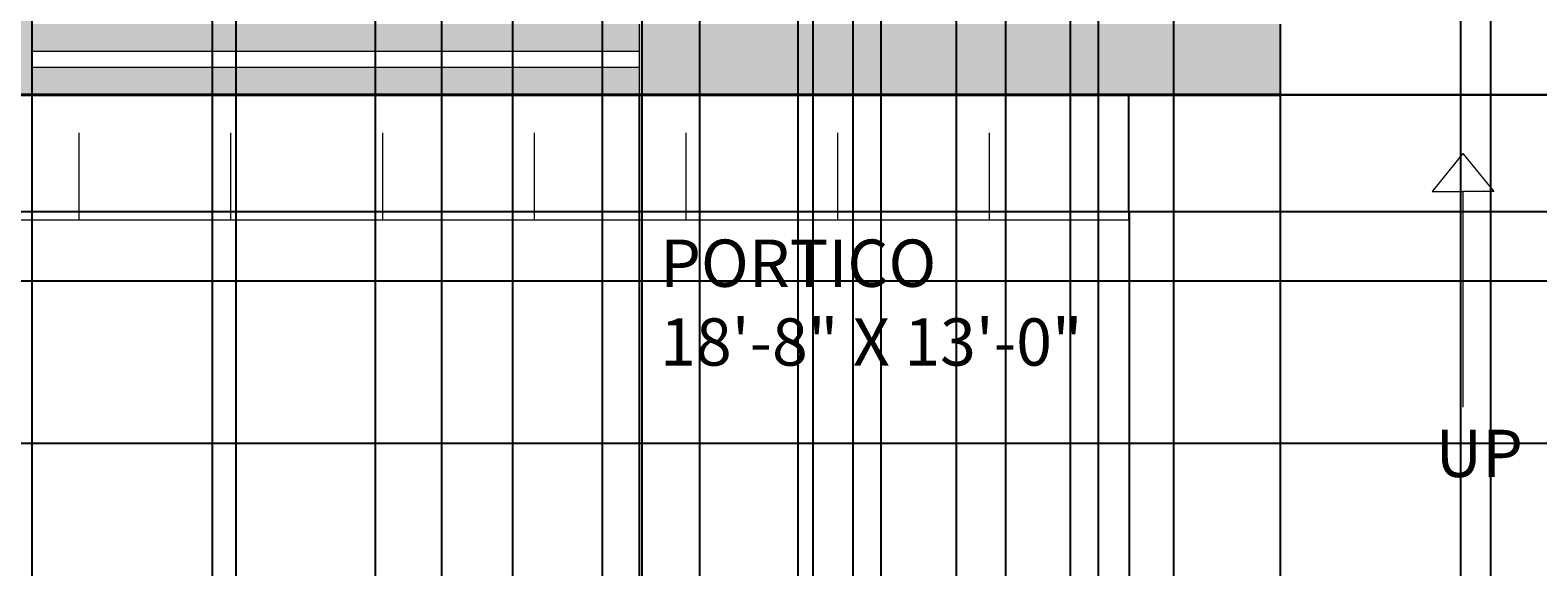
# Model space of a CAD drawing. Units: inches. Extents: x 818 to 1898, y 976 to 2364.
# Tile 22 of 96: x 1207 to 1398, y 1441 to 1509. Entities that reach past the tile are written whole.
import ezdxf

# ---------------------------------------------------------------- set-up
doc = ezdxf.new("R2010")
doc.units = ezdxf.units.IN
doc.header["$LTSCALE"] = 5
doc.header["$MEASUREMENT"] = 0
for name, color, linetype, lineweight in [('A-ANNO-DIMS', 2, 'Continuous', 18), ('A-ANNO-SYMB', 7, 'Continuous', 18), ('A-ANNO-TEXT', 7, 'Continuous', 18), ('A-AREA-IDEN', 7, 'Continuous', 18), ('A-DOOR', 3, 'Continuous', 25), ('A-FLOR-STRS', 7, 'Continuous', 25), ('A-GLAZ', 4, 'Continuous', 18), ('A-WALL', 7, 'Continuous', 40), ('C-PKNG', 8, 'Continuous', 18), ('C-PKNG-PATT', 9, 'Continuous', 9)]:
    doc.layers.add(name, color=color, linetype=linetype, lineweight=lineweight)
doc.layers.add('A-GLAZ-PATT', color=141, linetype='Continuous', lineweight=9, true_color=0xadddf7)
doc.layers.add('A-WALL-PATT', color=251, linetype='Continuous', lineweight=13, true_color=0x636466)
doc.styles.get("Standard").update_dxf_attribs({"font": 'arial.ttf'})
doc.dimstyles.get("Standard").update_dxf_attribs({"dimtxt": 0.18, "dimasz": 0.18, "dimexe": 0.18, "dimexo": 0.0625, "dimgap": 0.09, "dimtad": 0, "dimtih": 1, "dimtoh": 1, "dimdec": 4, "dimzin": 0, "dimdsep": 46, "dimtxsty": 'Standard', "dimcen": 0.09, "dimadec": 0, "dimazin": 0, "dimtfac": 1, "dimtdec": 4, "dimtofl": 0, "dimtmove": 0, "dimatfit": 3, "dimfxl": 1, "dimtolj": 1, "dimtzin": 0, "dimarcsym": 0})
pattern_1 = [(0, (0, 0), (0, 19.25), [14, -5.25]), (90, (0, 0), (-19.25, 1e-15), [14, -5.25])]

# ---------------------------------------------------------------- blocks, each defined once
blk = doc.blocks.new('*D59')
at = {"layer": 'A-ANNO-DIMS', "color": 0, "lineweight": -2, "ltscale": 5, "transparency": 16777216}
for p, q in [((1251.64, 2300.39), (818.03, 2300.39)), ((818.21, 2300.21), (818.21, 1669.95)), ((818.21, 1039.32), (818.21, 1669.59)), ((896.05, 1039.14), (818.03, 1039.14))]:
    blk.add_line(p, q, dxfattribs=at)
at = {"layer": 'A-ANNO-DIMS', "color": 0, "ltscale": 5, "transparency": 16777216}
for points in [[(818.18, 2300.21), (818.24, 2300.21), (818.21, 2300.39)], [(818.18, 1039.32), (818.24, 1039.32), (818.21, 1039.14)]]:
    blk.add_solid(points, dxfattribs=at)
at = {"layer": 'Defpoints', "color": 0, "ltscale": 5, "transparency": 16777216}
for p in [(818.21, 2300.39), (1251.71, 2300.39), (896.11, 1039.14)]:
    blk.add_point(p, dxfattribs=at)
at = {"layer": 'A-ANNO-DIMS', "color": 0, "ltscale": 5, "transparency": 16777216, "insert": (818.21, 1669.77), "char_height": 0.18, "attachment_point": 5}
blk.add_mtext('\\A1;1261.2', dxfattribs=at)
blk = doc.blocks.new('*D61')
at = {"layer": 'A-ANNO-DIMS', "color": 0, "lineweight": -2, "ltscale": 5, "transparency": 16777216}
for p, q in [((1071.73, 1203.03), (1071.73, 2363.87)), ((1071.91, 2363.69), (1250.94, 2363.69)), ((1430.55, 2363.69), (1251.51, 2363.69)), ((1430.73, 1203.03), (1430.73, 2363.87))]:
    blk.add_line(p, q, dxfattribs=at)
at = {"layer": 'A-ANNO-DIMS', "color": 0, "ltscale": 5, "transparency": 16777216}
for points in [[(1071.91, 2363.72), (1071.91, 2363.66), (1071.73, 2363.69)], [(1430.55, 2363.72), (1430.55, 2363.66), (1430.73, 2363.69)]]:
    blk.add_solid(points, dxfattribs=at)
at = {"layer": 'Defpoints', "color": 0, "ltscale": 5, "transparency": 16777216}
for p in [(1430.73, 2363.69), (1071.73, 1202.96), (1430.73, 1202.96)]:
    blk.add_point(p, dxfattribs=at)
at = {"layer": 'A-ANNO-DIMS', "color": 0, "ltscale": 5, "transparency": 16777216, "insert": (1251.23, 2363.69), "char_height": 0.18, "attachment_point": 5}
blk.add_mtext('\\A1;359', dxfattribs=at)
blk = doc.blocks.new('*D64')
at = {"layer": 'A-ANNO-DIMS', "color": 0, "lineweight": -2, "ltscale": 5, "transparency": 16777216}
for p, q in [((1197.73, 1501.14), (1197.73, 2363.87)), ((1197.91, 2363.69), (1313.93, 2363.69)), ((1430.55, 2363.69), (1314.52, 2363.69)), ((1430.73, 1501.14), (1430.73, 2363.87))]:
    blk.add_line(p, q, dxfattribs=at)
at = {"layer": 'A-ANNO-DIMS', "color": 0, "ltscale": 5, "transparency": 16777216}
for points in [[(1197.91, 2363.72), (1197.91, 2363.66), (1197.73, 2363.69)], [(1430.55, 2363.72), (1430.55, 2363.66), (1430.73, 2363.69)]]:
    blk.add_solid(points, dxfattribs=at)
at = {"layer": 'Defpoints', "color": 0, "ltscale": 5, "transparency": 16777216}
for p in [(1430.73, 2363.69), (1197.73, 1501.08), (1430.73, 1501.08)]:
    blk.add_point(p, dxfattribs=at)
at = {"layer": 'A-ANNO-DIMS', "color": 0, "ltscale": 5, "transparency": 16777216, "insert": (1314.23, 2363.69), "char_height": 0.18, "attachment_point": 5}
blk.add_mtext('\\A1;233', dxfattribs=at)
blk = doc.blocks.new('*D95')
at = {"layer": 'A-ANNO-DIMS', "color": 0, "lineweight": -2, "ltscale": 5, "transparency": 16777216}
for p, q in [((1173.54, 1071.12), (1173.54, 2363.87)), ((1173.72, 2363.69), (1201.29, 2363.69)), ((1229.47, 2363.69), (1201.9, 2363.69)), ((1229.65, 1071.12), (1229.65, 2363.87))]:
    blk.add_line(p, q, dxfattribs=at)
at = {"layer": 'A-ANNO-DIMS', "color": 0, "ltscale": 5, "transparency": 16777216}
for points in [[(1173.72, 2363.72), (1173.72, 2363.66), (1173.54, 2363.69)], [(1229.47, 2363.72), (1229.47, 2363.66), (1229.65, 2363.69)]]:
    blk.add_solid(points, dxfattribs=at)
at = {"layer": 'Defpoints', "color": 0, "ltscale": 5, "transparency": 16777216}
for p in [(1229.65, 2363.69), (1173.54, 1071.06), (1229.65, 1071.06)]:
    blk.add_point(p, dxfattribs=at)
at = {"layer": 'A-ANNO-DIMS', "color": 0, "ltscale": 5, "transparency": 16777216, "insert": (1201.59, 2363.69), "char_height": 0.18, "attachment_point": 5}
blk.add_mtext('\\A1;56.1', dxfattribs=at)
blk = doc.blocks.new('*D96')
at = {"layer": 'A-ANNO-DIMS', "color": 0, "lineweight": -2, "ltscale": 5, "transparency": 16777216}
for p, q in [((1229.65, 1071.12), (1229.65, 2363.87)), ((1229.83, 2363.69), (1256.52, 2363.69)), ((1283.99, 2363.69), (1257.3, 2363.69)), ((1284.17, 1071.12), (1284.17, 2363.87))]:
    blk.add_line(p, q, dxfattribs=at)
at = {"layer": 'A-ANNO-DIMS', "color": 0, "ltscale": 5, "transparency": 16777216}
for points in [[(1229.83, 2363.72), (1229.83, 2363.66), (1229.65, 2363.69)], [(1283.99, 2363.72), (1283.99, 2363.66), (1284.17, 2363.69)]]:
    blk.add_solid(points, dxfattribs=at)
at = {"layer": 'Defpoints', "color": 0, "ltscale": 5, "transparency": 16777216}
for p in [(1284.17, 2363.69), (1229.65, 1071.06), (1284.17, 1071.06)]:
    blk.add_point(p, dxfattribs=at)
at = {"layer": 'A-ANNO-DIMS', "color": 0, "ltscale": 5, "transparency": 16777216, "insert": (1256.91, 2363.69), "char_height": 0.18, "attachment_point": 5}
blk.add_mtext('\\A1;54.52', dxfattribs=at)
blk = doc.blocks.new('*D97')
at = {"layer": 'A-ANNO-DIMS', "color": 0, "lineweight": -2, "ltscale": 5, "transparency": 16777216}
for p, q in [((1284.17, 1071.12), (1284.17, 2363.87)), ((1284.35, 2363.69), (1310.96, 2363.69)), ((1338.36, 2363.69), (1311.75, 2363.69)), ((1338.54, 1071.12), (1338.54, 2363.87))]:
    blk.add_line(p, q, dxfattribs=at)
at = {"layer": 'A-ANNO-DIMS', "color": 0, "ltscale": 5, "transparency": 16777216}
for points in [[(1284.35, 2363.72), (1284.35, 2363.66), (1284.17, 2363.69)], [(1338.36, 2363.72), (1338.36, 2363.66), (1338.54, 2363.69)]]:
    blk.add_solid(points, dxfattribs=at)
at = {"layer": 'Defpoints', "color": 0, "ltscale": 5, "transparency": 16777216}
for p in [(1338.54, 2363.69), (1284.17, 1071.06), (1338.54, 1071.06)]:
    blk.add_point(p, dxfattribs=at)
at = {"layer": 'A-ANNO-DIMS', "color": 0, "ltscale": 5, "transparency": 16777216, "insert": (1311.36, 2363.69), "char_height": 0.18, "attachment_point": 5}
blk.add_mtext('\\A1;54.37', dxfattribs=at)
blk = doc.blocks.new('*D98')
at = {"layer": 'A-ANNO-DIMS', "color": 0, "lineweight": -2, "ltscale": 5, "transparency": 16777216}
for p, q in [((1338.54, 1071.12), (1338.54, 2363.87)), ((1338.72, 2363.69), (1364.81, 2363.69)), ((1391.7, 2363.69), (1365.6, 2363.69)), ((1391.88, 1071.12), (1391.88, 2363.87))]:
    blk.add_line(p, q, dxfattribs=at)
at = {"layer": 'A-ANNO-DIMS', "color": 0, "ltscale": 5, "transparency": 16777216}
for points in [[(1338.72, 2363.72), (1338.72, 2363.66), (1338.54, 2363.69)], [(1391.7, 2363.72), (1391.7, 2363.66), (1391.88, 2363.69)]]:
    blk.add_solid(points, dxfattribs=at)
at = {"layer": 'Defpoints', "color": 0, "ltscale": 5, "transparency": 16777216}
for p in [(1391.88, 2363.69), (1338.54, 1071.06), (1391.88, 1071.06)]:
    blk.add_point(p, dxfattribs=at)
at = {"layer": 'A-ANNO-DIMS', "color": 0, "ltscale": 5, "transparency": 16777216, "insert": (1365.21, 2363.69), "char_height": 0.18, "attachment_point": 5}
blk.add_mtext('\\A1;53.33', dxfattribs=at)
blk = doc.blocks.new('*D99')
at = {"layer": 'A-ANNO-DIMS', "color": 0, "lineweight": -2, "ltscale": 5, "transparency": 16777216}
for p, q in [((1391.88, 1071.12), (1391.88, 2363.87)), ((1392.06, 2363.69), (1420.45, 2363.69)), ((1449.64, 2363.69), (1421.24, 2363.69)), ((1449.82, 1071.12), (1449.82, 2363.87))]:
    blk.add_line(p, q, dxfattribs=at)
at = {"layer": 'A-ANNO-DIMS', "color": 0, "ltscale": 5, "transparency": 16777216}
for points in [[(1392.06, 2363.72), (1392.06, 2363.66), (1391.88, 2363.69)], [(1449.64, 2363.72), (1449.64, 2363.66), (1449.82, 2363.69)]]:
    blk.add_solid(points, dxfattribs=at)
at = {"layer": 'Defpoints', "color": 0, "ltscale": 5, "transparency": 16777216}
for p in [(1449.82, 2363.69), (1391.88, 1071.06), (1449.82, 1071.06)]:
    blk.add_point(p, dxfattribs=at)
at = {"layer": 'A-ANNO-DIMS', "color": 0, "ltscale": 5, "transparency": 16777216, "insert": (1420.85, 2363.69), "char_height": 0.18, "attachment_point": 5}
blk.add_mtext('\\A1;57.94', dxfattribs=at)
blk = doc.blocks.new('*D116')
at = {"layer": 'A-ANNO-DIMS', "color": 0, "lineweight": -2, "ltscale": 5, "transparency": 16777216}
for p, q in [((1766.29, 1456.81), (818.03, 1456.81)), ((818.21, 1456.63), (818.21, 1417.41)), ((818.21, 1377.84), (818.21, 1417.05)), ((1766.29, 1377.66), (818.03, 1377.66))]:
    blk.add_line(p, q, dxfattribs=at)
at = {"layer": 'A-ANNO-DIMS', "color": 0, "ltscale": 5, "transparency": 16777216}
for points in [[(818.18, 1456.63), (818.24, 1456.63), (818.21, 1456.81)], [(818.18, 1377.84), (818.24, 1377.84), (818.21, 1377.66)]]:
    blk.add_solid(points, dxfattribs=at)
at = {"layer": 'Defpoints', "color": 0, "ltscale": 5, "transparency": 16777216}
for p in [(818.21, 1456.81), (1766.35, 1456.81), (1766.35, 1377.66)]:
    blk.add_point(p, dxfattribs=at)
at = {"layer": 'A-ANNO-DIMS', "color": 0, "ltscale": 5, "transparency": 16777216, "insert": (818.21, 1417.23), "char_height": 0.18, "attachment_point": 5}
blk.add_mtext('\\A1;79.15', dxfattribs=at)
blk = doc.blocks.new('*D117')
at = {"layer": 'A-ANNO-DIMS', "color": 0, "lineweight": -2, "ltscale": 5, "transparency": 16777216}
for p, q in [((1766.29, 1545.18), (818.03, 1545.18)), ((818.21, 1545), (818.21, 1501.18)), ((818.21, 1456.99), (818.21, 1500.81)), ((1766.29, 1456.81), (818.03, 1456.81))]:
    blk.add_line(p, q, dxfattribs=at)
at = {"layer": 'A-ANNO-DIMS', "color": 0, "ltscale": 5, "transparency": 16777216}
for points in [[(818.18, 1545), (818.24, 1545), (818.21, 1545.18)], [(818.18, 1456.99), (818.24, 1456.99), (818.21, 1456.81)]]:
    blk.add_solid(points, dxfattribs=at)
at = {"layer": 'Defpoints', "color": 0, "ltscale": 5, "transparency": 16777216}
for p in [(818.21, 1545.18), (1766.35, 1545.18), (1766.35, 1456.81)]:
    blk.add_point(p, dxfattribs=at)
at = {"layer": 'A-ANNO-DIMS', "color": 0, "ltscale": 5, "transparency": 16777216, "insert": (818.21, 1501), "char_height": 0.18, "attachment_point": 5}
blk.add_mtext('\\A1;88.37', dxfattribs=at)
blk = doc.blocks.new('*D145')
at = {"layer": 'A-ANNO-DIMS', "color": 0, "lineweight": -2, "ltscale": 5, "transparency": 16777216}
for p, q in [((1197.39, 2122.31), (1197.39, 975.66)), ((1232.61, 2122.31), (1232.61, 975.66)), ((1197.57, 975.84), (1214.61, 975.84)), ((1232.43, 975.84), (1215.39, 975.84))]:
    blk.add_line(p, q, dxfattribs=at)
at = {"layer": 'A-ANNO-DIMS', "color": 0, "ltscale": 5, "transparency": 16777216}
for points in [[(1197.57, 975.87), (1197.57, 975.81), (1197.39, 975.84)], [(1232.43, 975.87), (1232.43, 975.81), (1232.61, 975.84)]]:
    blk.add_solid(points, dxfattribs=at)
at = {"layer": 'Defpoints', "color": 0, "ltscale": 5, "transparency": 16777216}
for p in [(1197.39, 2122.38), (1232.61, 2122.38), (1232.61, 975.84)]:
    blk.add_point(p, dxfattribs=at)
at = {"layer": 'A-ANNO-DIMS', "color": 0, "ltscale": 5, "transparency": 16777216, "insert": (1215, 975.84), "char_height": 0.18, "attachment_point": 5}
blk.add_mtext('\\A1;35.22', dxfattribs=at)
blk = doc.blocks.new('*D159')
at = {"layer": 'A-ANNO-DIMS', "color": 0, "lineweight": -2, "ltscale": 5, "transparency": 16777216}
for p, q in [((1206.73, 1687.02), (1206.73, 975.66)), ((1463.73, 1687.02), (1463.73, 975.66)), ((1206.91, 975.84), (1334.93, 975.84)), ((1463.55, 975.84), (1335.52, 975.84))]:
    blk.add_line(p, q, dxfattribs=at)
at = {"layer": 'A-ANNO-DIMS', "color": 0, "ltscale": 5, "transparency": 16777216}
for points in [[(1206.91, 975.87), (1206.91, 975.81), (1206.73, 975.84)], [(1463.55, 975.87), (1463.55, 975.81), (1463.73, 975.84)]]:
    blk.add_solid(points, dxfattribs=at)
at = {"layer": 'Defpoints', "color": 0, "ltscale": 5, "transparency": 16777216}
for p in [(1206.73, 1687.08), (1463.73, 1687.08), (1463.73, 975.84)]:
    blk.add_point(p, dxfattribs=at)
at = {"layer": 'A-ANNO-DIMS', "color": 0, "ltscale": 5, "transparency": 16777216, "insert": (1335.23, 975.84), "char_height": 0.18, "attachment_point": 5}
blk.add_mtext('\\A1;257', dxfattribs=at)
blk = doc.blocks.new('*D163')
at = {"layer": 'A-ANNO-DIMS', "color": 0, "lineweight": -2, "ltscale": 5, "transparency": 16777216}
for p, q in [((1365.15, 1501.02), (1365.15, 975.66)), ((1401.15, 1501.02), (1401.15, 975.66)), ((1365.33, 975.84), (1382.93, 975.84)), ((1400.97, 975.84), (1383.37, 975.84))]:
    blk.add_line(p, q, dxfattribs=at)
at = {"layer": 'A-ANNO-DIMS', "color": 0, "ltscale": 5, "transparency": 16777216}
for points in [[(1365.33, 975.87), (1365.33, 975.81), (1365.15, 975.84)], [(1400.97, 975.87), (1400.97, 975.81), (1401.15, 975.84)]]:
    blk.add_solid(points, dxfattribs=at)
at = {"layer": 'Defpoints', "color": 0, "ltscale": 5, "transparency": 16777216}
for p in [(1365.15, 1501.08), (1401.15, 1501.08), (1401.15, 975.84)]:
    blk.add_point(p, dxfattribs=at)
at = {"layer": 'A-ANNO-DIMS', "color": 0, "ltscale": 5, "transparency": 16777216, "insert": (1383.15, 975.84), "char_height": 0.18, "attachment_point": 5}
blk.add_mtext('\\A1;36', dxfattribs=at)
blk = doc.blocks.new('*D164')
at = {"layer": 'A-ANNO-DIMS', "color": 0, "lineweight": -2, "ltscale": 5, "transparency": 16777216}
for p, q in [((1206.73, 1501.02), (1206.73, 975.66)), ((1283.82, 1501.02), (1283.82, 975.66)), ((1206.91, 975.84), (1244.97, 975.84)), ((1283.64, 975.84), (1245.58, 975.84))]:
    blk.add_line(p, q, dxfattribs=at)
at = {"layer": 'A-ANNO-DIMS', "color": 0, "ltscale": 5, "transparency": 16777216}
for points in [[(1206.91, 975.87), (1206.91, 975.81), (1206.73, 975.84)], [(1283.64, 975.87), (1283.64, 975.81), (1283.82, 975.84)]]:
    blk.add_solid(points, dxfattribs=at)
at = {"layer": 'Defpoints', "color": 0, "ltscale": 5, "transparency": 16777216}
for p in [(1206.73, 1501.08), (1283.82, 1501.08), (1283.82, 975.84)]:
    blk.add_point(p, dxfattribs=at)
at = {"layer": 'A-ANNO-DIMS', "color": 0, "ltscale": 5, "transparency": 16777216, "insert": (1245.27, 975.84), "char_height": 0.18, "attachment_point": 5}
blk.add_mtext('\\A1;77.1', dxfattribs=at)
blk = doc.blocks.new('*D167')
at = {"layer": 'A-ANNO-DIMS', "color": 0, "lineweight": -2, "ltscale": 5, "transparency": 16777216}
for p, q in [((1345.97, 1486.18), (1345.97, 975.66)), ((1430.73, 1486.18), (1430.73, 975.66)), ((1346.15, 975.84), (1387.95, 975.84)), ((1430.55, 975.84), (1388.74, 975.84))]:
    blk.add_line(p, q, dxfattribs=at)
at = {"layer": 'A-ANNO-DIMS', "color": 0, "ltscale": 5, "transparency": 16777216}
for points in [[(1346.15, 975.87), (1346.15, 975.81), (1345.97, 975.84)], [(1430.55, 975.87), (1430.55, 975.81), (1430.73, 975.84)]]:
    blk.add_solid(points, dxfattribs=at)
at = {"layer": 'Defpoints', "color": 0, "ltscale": 5, "transparency": 16777216}
for p in [(1345.97, 1486.24), (1430.73, 1486.24), (1430.73, 975.84)]:
    blk.add_point(p, dxfattribs=at)
at = {"layer": 'A-ANNO-DIMS', "color": 0, "ltscale": 5, "transparency": 16777216, "insert": (1388.35, 975.84), "char_height": 0.18, "attachment_point": 5}
blk.add_mtext('\\A1;84.76', dxfattribs=at)
blk = doc.blocks.new('*D168')
at = {"layer": 'A-ANNO-DIMS', "color": 0, "lineweight": -2, "ltscale": 5, "transparency": 16777216}
for p, q in [((1430.66, 1501.08), (818.03, 1501.08)), ((818.21, 1500.9), (818.21, 1493.84)), ((818.21, 1486.42), (818.21, 1493.48)), ((1430.66, 1486.24), (818.03, 1486.24))]:
    blk.add_line(p, q, dxfattribs=at)
at = {"layer": 'A-ANNO-DIMS', "color": 0, "ltscale": 5, "transparency": 16777216}
for points in [[(818.18, 1500.9), (818.24, 1500.9), (818.21, 1501.08)], [(818.18, 1486.42), (818.24, 1486.42), (818.21, 1486.24)]]:
    blk.add_solid(points, dxfattribs=at)
at = {"layer": 'Defpoints', "color": 0, "ltscale": 5, "transparency": 16777216}
for p in [(818.21, 1501.08), (1430.73, 1501.08), (1430.73, 1486.24)]:
    blk.add_point(p, dxfattribs=at)
at = {"layer": 'A-ANNO-DIMS', "color": 0, "ltscale": 5, "transparency": 16777216, "insert": (818.21, 1493.66), "char_height": 0.18, "attachment_point": 5}
blk.add_mtext('\\A1;14.84', dxfattribs=at)
blk = doc.blocks.new('*D201')
at = {"layer": 'A-ANNO-DIMS', "color": 0, "lineweight": -2, "ltscale": 5, "transparency": 16777216}
for p, q in [((1678.27, 1518.56), (818.03, 1518.56)), ((818.21, 1518.38), (818.21, 1498.18)), ((818.21, 1477.61), (818.21, 1497.81)), ((1678.27, 1477.43), (818.03, 1477.43))]:
    blk.add_line(p, q, dxfattribs=at)
at = {"layer": 'A-ANNO-DIMS', "color": 0, "ltscale": 5, "transparency": 16777216}
for points in [[(818.18, 1518.38), (818.24, 1518.38), (818.21, 1518.56)], [(818.18, 1477.61), (818.24, 1477.61), (818.21, 1477.43)]]:
    blk.add_solid(points, dxfattribs=at)
at = {"layer": 'Defpoints', "color": 0, "ltscale": 5, "transparency": 16777216}
for p in [(818.21, 1518.56), (1678.33, 1518.56), (1678.33, 1477.43)]:
    blk.add_point(p, dxfattribs=at)
at = {"layer": 'A-ANNO-DIMS', "color": 0, "ltscale": 5, "transparency": 16777216, "insert": (818.21, 1497.99), "char_height": 0.18, "attachment_point": 5}
blk.add_mtext('\\A1;41.135', dxfattribs=at)
blk = doc.blocks.new('*D231')
at = {"layer": 'A-ANNO-DIMS', "color": 0, "lineweight": -2, "ltscale": 5, "transparency": 16777216}
for p, q in [((1303.93, 1952.98), (1303.93, 975.66)), ((1402.52, 1952.98), (1402.52, 975.66)), ((1304.11, 975.84), (1352.83, 975.84)), ((1402.34, 975.84), (1353.62, 975.84))]:
    blk.add_line(p, q, dxfattribs=at)
at = {"layer": 'A-ANNO-DIMS', "color": 0, "ltscale": 5, "transparency": 16777216}
for points in [[(1304.11, 975.87), (1304.11, 975.81), (1303.93, 975.84)], [(1402.34, 975.87), (1402.34, 975.81), (1402.52, 975.84)]]:
    blk.add_solid(points, dxfattribs=at)
at = {"layer": 'Defpoints', "color": 0, "ltscale": 5, "transparency": 16777216}
for p in [(1303.93, 1953.04), (1402.52, 1953.04), (1402.52, 975.84)]:
    blk.add_point(p, dxfattribs=at)
at = {"layer": 'A-ANNO-DIMS', "color": 0, "ltscale": 5, "transparency": 16777216, "insert": (1353.22, 975.84), "char_height": 0.18, "attachment_point": 5}
blk.add_mtext('\\A1;98.59', dxfattribs=at)
blk = doc.blocks.new('*D233')
at = {"layer": 'A-ANNO-DIMS', "color": 0, "lineweight": -2, "ltscale": 5, "transparency": 16777216}
for p, q in [((1267.73, 2044.02), (1267.73, 975.66)), ((1303.93, 2008.33), (1303.93, 975.66)), ((1267.91, 975.84), (1285.36, 975.84)), ((1303.75, 975.84), (1286.29, 975.84))]:
    blk.add_line(p, q, dxfattribs=at)
at = {"layer": 'A-ANNO-DIMS', "color": 0, "ltscale": 5, "transparency": 16777216}
for points in [[(1267.91, 975.87), (1267.91, 975.81), (1267.73, 975.84)], [(1303.75, 975.87), (1303.75, 975.81), (1303.93, 975.84)]]:
    blk.add_solid(points, dxfattribs=at)
at = {"layer": 'Defpoints', "color": 0, "ltscale": 5, "transparency": 16777216}
for p in [(1267.73, 2044.08), (1303.93, 2008.39), (1303.93, 975.84)]:
    blk.add_point(p, dxfattribs=at)
at = {"layer": 'A-ANNO-DIMS', "color": 0, "ltscale": 5, "transparency": 16777216, "insert": (1285.83, 975.84), "char_height": 0.18, "attachment_point": 5}
blk.add_mtext('\\A1;36.206', dxfattribs=at)
blk = doc.blocks.new('*D236')
at = {"layer": 'A-ANNO-DIMS', "color": 0, "lineweight": -2, "ltscale": 5, "transparency": 16777216}
for p, q in [((1310.91, 2026.14), (1310.91, 975.66)), ((1342.04, 2026.14), (1342.04, 975.66)), ((1311.09, 975.84), (1326.08, 975.84)), ((1341.86, 975.84), (1326.87, 975.84))]:
    blk.add_line(p, q, dxfattribs=at)
at = {"layer": 'A-ANNO-DIMS', "color": 0, "ltscale": 5, "transparency": 16777216}
for points in [[(1311.09, 975.87), (1311.09, 975.81), (1310.91, 975.84)], [(1341.86, 975.87), (1341.86, 975.81), (1342.04, 975.84)]]:
    blk.add_solid(points, dxfattribs=at)
at = {"layer": 'Defpoints', "color": 0, "ltscale": 5, "transparency": 16777216}
for p in [(1310.91, 2026.21), (1342.04, 2026.21), (1342.04, 975.84)]:
    blk.add_point(p, dxfattribs=at)
at = {"layer": 'A-ANNO-DIMS', "color": 0, "ltscale": 5, "transparency": 16777216, "insert": (1326.48, 975.84), "char_height": 0.18, "attachment_point": 5}
blk.add_mtext('\\A1;31.14', dxfattribs=at)
blk = doc.blocks.new('*D245')
at = {"layer": 'A-ANNO-DIMS', "color": 0, "lineweight": -2, "ltscale": 5, "transparency": 16777216}
for p, q in [((1291.48, 1599.31), (1291.48, 975.66)), ((1314.49, 1599.31), (1314.49, 975.66)), ((1291.66, 975.84), (1302.61, 975.84)), ((1314.31, 975.84), (1303.36, 975.84))]:
    blk.add_line(p, q, dxfattribs=at)
at = {"layer": 'A-ANNO-DIMS', "color": 0, "ltscale": 5, "transparency": 16777216}
for points in [[(1291.66, 975.87), (1291.66, 975.81), (1291.48, 975.84)], [(1314.31, 975.87), (1314.31, 975.81), (1314.49, 975.84)]]:
    blk.add_solid(points, dxfattribs=at)
at = {"layer": 'Defpoints', "color": 0, "ltscale": 5, "transparency": 16777216}
for p in [(1291.48, 1599.37), (1314.49, 1599.37), (1314.49, 975.84)]:
    blk.add_point(p, dxfattribs=at)
at = {"layer": 'A-ANNO-DIMS', "color": 0, "ltscale": 5, "transparency": 16777216, "insert": (1302.98, 975.84), "char_height": 0.18, "attachment_point": 5}
blk.add_mtext('\\A1;23.01', dxfattribs=at)
blk = doc.blocks.new('*D251')
at = {"layer": 'A-ANNO-DIMS', "color": 0, "lineweight": -2, "ltscale": 5, "transparency": 16777216}
for p, q in [((1250.3, 1878.33), (1250.3, 975.66)), ((1258.73, 1878.33), (1258.73, 975.66)), ((1250.48, 975.84), (1254.12, 975.84)), ((1258.55, 975.84), (1254.91, 975.84))]:
    blk.add_line(p, q, dxfattribs=at)
at = {"layer": 'A-ANNO-DIMS', "color": 0, "ltscale": 5, "transparency": 16777216}
for points in [[(1250.48, 975.87), (1250.48, 975.81), (1250.3, 975.84)], [(1258.55, 975.87), (1258.55, 975.81), (1258.73, 975.84)]]:
    blk.add_solid(points, dxfattribs=at)
at = {"layer": 'Defpoints', "color": 0, "ltscale": 5, "transparency": 16777216}
for p in [(1250.3, 1878.39), (1258.73, 1878.39), (1258.73, 975.84)]:
    blk.add_point(p, dxfattribs=at)
at = {"layer": 'A-ANNO-DIMS', "color": 0, "ltscale": 5, "transparency": 16777216, "insert": (1254.51, 975.84), "char_height": 0.18, "attachment_point": 5}
blk.add_mtext('\\A1;8.422', dxfattribs=at)
blk = doc.blocks.new('*D252')
at = {"layer": 'A-ANNO-DIMS', "color": 0, "lineweight": -2, "ltscale": 5, "transparency": 16777216}
for p, q in [((1330.3, 2053.02), (1330.3, 975.66)), ((1388.03, 2053.02), (1388.03, 975.66)), ((1330.48, 975.84), (1358.77, 975.84)), ((1387.85, 975.84), (1359.56, 975.84))]:
    blk.add_line(p, q, dxfattribs=at)
at = {"layer": 'A-ANNO-DIMS', "color": 0, "ltscale": 5, "transparency": 16777216}
for points in [[(1330.48, 975.87), (1330.48, 975.81), (1330.3, 975.84)], [(1387.85, 975.87), (1387.85, 975.81), (1388.03, 975.84)]]:
    blk.add_solid(points, dxfattribs=at)
at = {"layer": 'Defpoints', "color": 0, "ltscale": 5, "transparency": 16777216}
for p in [(1330.3, 2053.08), (1388.03, 2053.08), (1388.03, 975.84)]:
    blk.add_point(p, dxfattribs=at)
at = {"layer": 'A-ANNO-DIMS', "color": 0, "ltscale": 5, "transparency": 16777216, "insert": (1359.17, 975.84), "char_height": 0.18, "attachment_point": 5}
blk.add_mtext('\\A1;57.73', dxfattribs=at)
blk = doc.blocks.new('*D254')
at = {"layer": 'A-ANNO-DIMS', "color": 0, "lineweight": -2, "ltscale": 5, "transparency": 16777216}
for p, q in [((1267.73, 2044.02), (1267.73, 975.66)), ((1330.3, 2044.02), (1330.3, 975.66)), ((1267.91, 975.84), (1298.62, 975.84)), ((1330.12, 975.84), (1299.41, 975.84))]:
    blk.add_line(p, q, dxfattribs=at)
at = {"layer": 'A-ANNO-DIMS', "color": 0, "ltscale": 5, "transparency": 16777216}
for points in [[(1267.91, 975.87), (1267.91, 975.81), (1267.73, 975.84)], [(1330.12, 975.87), (1330.12, 975.81), (1330.3, 975.84)]]:
    blk.add_solid(points, dxfattribs=at)
at = {"layer": 'Defpoints', "color": 0, "ltscale": 5, "transparency": 16777216}
for p in [(1267.73, 2044.08), (1330.3, 2044.08), (1330.3, 975.84)]:
    blk.add_point(p, dxfattribs=at)
at = {"layer": 'A-ANNO-DIMS', "color": 0, "ltscale": 5, "transparency": 16777216, "insert": (1299.02, 975.84), "char_height": 0.18, "attachment_point": 5}
blk.add_mtext('\\A1;62.58', dxfattribs=at)
blk = doc.blocks.new('*D278')
at = {"layer": 'A-ANNO-DIMS', "color": 0, "lineweight": -2, "ltscale": 5, "transparency": 16777216}
for p, q in [((1324.03, 1700.74), (1324.03, 975.66)), ((1267.73, 1696.02), (1267.73, 975.66)), ((1267.91, 975.84), (1295.5, 975.84)), ((1323.85, 975.84), (1296.26, 975.84))]:
    blk.add_line(p, q, dxfattribs=at)
at = {"layer": 'A-ANNO-DIMS', "color": 0, "ltscale": 5, "transparency": 16777216}
for points in [[(1267.91, 975.87), (1267.91, 975.81), (1267.73, 975.84)], [(1323.85, 975.87), (1323.85, 975.81), (1324.03, 975.84)]]:
    blk.add_solid(points, dxfattribs=at)
at = {"layer": 'Defpoints', "color": 0, "ltscale": 5, "transparency": 16777216}
for p in [(1324.03, 1700.81), (1267.73, 1696.08), (1324.03, 975.84)]:
    blk.add_point(p, dxfattribs=at)
at = {"layer": 'A-ANNO-DIMS', "color": 0, "ltscale": 5, "transparency": 16777216, "insert": (1295.88, 975.84), "char_height": 0.18, "attachment_point": 5}
blk.add_mtext('\\A1;56.31', dxfattribs=at)
blk = doc.blocks.new('*D279')
at = {"layer": 'A-ANNO-DIMS', "color": 0, "lineweight": -2, "ltscale": 5, "transparency": 16777216}
for p, q in [((1279.13, 1713.75), (1279.13, 975.66)), ((1267.73, 1696.02), (1267.73, 975.66)), ((1267.91, 975.84), (1273.11, 975.84)), ((1278.95, 975.84), (1273.74, 975.84))]:
    blk.add_line(p, q, dxfattribs=at)
at = {"layer": 'A-ANNO-DIMS', "color": 0, "ltscale": 5, "transparency": 16777216}
for points in [[(1267.91, 975.87), (1267.91, 975.81), (1267.73, 975.84)], [(1278.95, 975.87), (1278.95, 975.81), (1279.13, 975.84)]]:
    blk.add_solid(points, dxfattribs=at)
at = {"layer": 'Defpoints', "color": 0, "ltscale": 5, "transparency": 16777216}
for p in [(1279.13, 1713.82), (1267.73, 1696.08), (1267.73, 975.84)]:
    blk.add_point(p, dxfattribs=at)
at = {"layer": 'A-ANNO-DIMS', "color": 0, "ltscale": 5, "transparency": 16777216, "insert": (1273.43, 975.84), "char_height": 0.18, "attachment_point": 5}
blk.add_mtext('\\A1;11.4', dxfattribs=at)
blk = doc.blocks.new('*D283')
at = {"layer": 'A-ANNO-DIMS', "color": 0, "lineweight": -2, "ltscale": 5, "transparency": 16777216}
for p, q in [((1351.6, 1761.39), (1351.6, 975.66)), ((1267.73, 1696.02), (1267.73, 975.66)), ((1267.91, 975.84), (1309.27, 975.84)), ((1351.42, 975.84), (1310.06, 975.84))]:
    blk.add_line(p, q, dxfattribs=at)
at = {"layer": 'A-ANNO-DIMS', "color": 0, "ltscale": 5, "transparency": 16777216}
for points in [[(1267.91, 975.87), (1267.91, 975.81), (1267.73, 975.84)], [(1351.42, 975.87), (1351.42, 975.81), (1351.6, 975.84)]]:
    blk.add_solid(points, dxfattribs=at)
at = {"layer": 'Defpoints', "color": 0, "ltscale": 5, "transparency": 16777216}
for p in [(1351.6, 1761.45), (1267.73, 1696.08), (1351.6, 975.84)]:
    blk.add_point(p, dxfattribs=at)
at = {"layer": 'A-ANNO-DIMS', "color": 0, "ltscale": 5, "transparency": 16777216, "insert": (1309.66, 975.84), "char_height": 0.18, "attachment_point": 5}
blk.add_mtext('\\A1;83.87', dxfattribs=at)
blk = doc.blocks.new('*D285')
at = {"layer": 'A-ANNO-DIMS', "color": 0, "lineweight": -2, "ltscale": 5, "transparency": 16777216}
for p, q in [((1305.83, 1830.02), (1305.83, 975.66)), ((1267.73, 1814.9), (1267.73, 975.66)), ((1267.91, 975.84), (1286.47, 975.84)), ((1305.65, 975.84), (1287.08, 975.84))]:
    blk.add_line(p, q, dxfattribs=at)
at = {"layer": 'A-ANNO-DIMS', "color": 0, "ltscale": 5, "transparency": 16777216}
for points in [[(1267.91, 975.87), (1267.91, 975.81), (1267.73, 975.84)], [(1305.65, 975.87), (1305.65, 975.81), (1305.83, 975.84)]]:
    blk.add_solid(points, dxfattribs=at)
at = {"layer": 'Defpoints', "color": 0, "ltscale": 5, "transparency": 16777216}
for p in [(1305.83, 1830.08), (1267.73, 1814.97), (1267.73, 975.84)]:
    blk.add_point(p, dxfattribs=at)
at = {"layer": 'A-ANNO-DIMS', "color": 0, "ltscale": 5, "transparency": 16777216, "insert": (1286.78, 975.84), "char_height": 0.18, "attachment_point": 5}
blk.add_mtext('\\A1;38.1', dxfattribs=at)

msp = doc.modelspace()

# ---------------------------------------------------------------- hatches: boundary and pattern name
at = {"layer": 'A-GLAZ-PATT', "ltscale": 5}
h = msp.add_hatch(color=256, dxfattribs=at)
h.dxf.hatch_style = 1
h.paths.add_polyline_path([(1283.8183, 1504.5782), (1206.7251, 1504.5782), (1206.7251, 1501.0782), (1283.8183, 1501.0782)])
h.paths.add_polyline_path([(1283.8183, 1510.0782), (1206.7251, 1510.0782), (1206.7251, 1506.5782), (1283.8183, 1506.5782)])
h.paths.add_polyline_path([(1490.9163, 1355.0782), (1439.7252, 1355.0782), (1439.7252, 1409.0522), (1436.2252, 1409.0522), (1436.2252, 1351.5782), (1490.9163, 1351.5782)])
h.paths.add_polyline_path([(1434.2252, 1409.0522), (1430.7251, 1409.0522), (1430.7251, 1346.0782), (1435.0799, 1346.0782), (1435.0731, 1346.1152), (1435.1501, 1346.0782), (1490.9163, 1346.0782), (1490.9163, 1349.5782), (1434.2252, 1349.5782)])
h.paths.add_polyline_path([(1714.7252, 1545.0782), (1711.2252, 1545.0782), (1711.2252, 1521.0782), (1714.7252, 1521.0782)])
h.paths.add_polyline_path([(1709.2252, 1545.0782), (1705.7252, 1545.0782), (1705.7252, 1521.0782), (1709.2252, 1521.0782)])
h.paths.add_polyline_path([(1714.7252, 1687.0782), (1711.2252, 1687.0782), (1711.2252, 1649.9029), (1714.7252, 1649.9029)])
h.paths.add_polyline_path([(1709.2252, 1687.0782), (1705.7252, 1687.0782), (1705.7252, 1649.9029), (1709.2252, 1649.9029)])
h.paths.add_polyline_path([(1709.2252, 1745.5584), (1705.7252, 1745.5584), (1705.7252, 1717.3178), (1709.2252, 1717.3178)])
h.paths.add_polyline_path([(1714.7252, 1745.5584), (1711.2252, 1745.5584), (1711.2252, 1717.3178), (1714.7252, 1717.3178)])
h.paths.add_polyline_path([(1714.7252, 2014.5114), (1711.2252, 2014.5114), (1711.2252, 1962.0338), (1714.7252, 1962.0338)])
h.paths.add_polyline_path([(1709.2252, 2014.5114), (1705.7252, 2014.5114), (1705.7252, 1962.0338), (1709.2252, 1962.0338)])
h.paths.add_polyline_path([(1538.5155, 2047.5782), (1485.1216, 2047.5782), (1485.1216, 2044.0782), (1538.5155, 2044.0782)])
h.paths.add_polyline_path([(1538.5155, 2053.0782), (1485.1216, 2053.0782), (1485.1216, 2049.5782), (1538.5155, 2049.5782)])
h.paths.add_polyline_path([(1388.0315, 2047.5782), (1330.305, 2047.5782), (1330.305, 2044.0782), (1388.0315, 2044.0782)])
h.paths.add_polyline_path([(1388.0315, 2053.0782), (1330.305, 2053.0782), (1330.305, 2049.5782), (1388.0315, 2049.5782)])
h.paths.add_polyline_path([(1262.2252, 2019.2871), (1258.7251, 2019.2871), (1258.7251, 1928.9218), (1262.2252, 1928.9218)])
h.paths.add_polyline_path([(1267.7251, 2019.2871), (1264.2252, 2019.2871), (1264.2252, 1928.9218), (1267.7251, 1928.9218)])
h.paths.add_polyline_path([(1262.2252, 1862.9652), (1258.7251, 1862.9652), (1258.7251, 1814.9652), (1262.2252, 1814.9652)])
h.paths.add_polyline_path([(1267.7251, 1862.9652), (1264.2252, 1862.9652), (1264.2252, 1814.9652), (1267.7251, 1814.9652)])
h.paths.add_polyline_path([(1262.2252, 1755.3321), (1258.7251, 1755.3321), (1258.7251, 1707.3321), (1262.2252, 1707.3321)])
h.paths.add_polyline_path([(1267.7251, 1755.3321), (1264.2252, 1755.3321), (1264.2252, 1707.3321), (1267.7251, 1707.3321)])
h.paths.add_polyline_path([(1251.9333, 1692.5782), (1206.7251, 1692.5782), (1206.7251, 1687.0782), (1251.9333, 1687.0782)])
h.paths.add_polyline_path([(1251.9333, 1700.0782), (1206.7251, 1700.0782), (1206.7251, 1694.5782), (1251.9333, 1694.5782)])
at = {"layer": 'A-WALL-PATT', "ltscale": 5}
h = msp.add_hatch(color=256, dxfattribs=at)
h.dxf.hatch_style = 1
h.paths.add_polyline_path([(1206.7251, 1687.0782), (1206.7251, 1700.0782), (1197.7251, 1700.0782), (1197.7251, 1501.0782), (1206.7251, 1501.0782), (1206.7251, 1510.0782)])
h.paths.add_polyline_path([(1197.7251, 1590.7585), (1173.7252, 1590.7585), (1173.7252, 1586.7585), (1197.7251, 1586.7585)])
h.paths.add_polyline_path([(1197.7251, 1534.6024), (1173.7252, 1534.6024), (1173.7252, 1530.6024), (1197.7251, 1530.6024)])
h.paths.add_polyline_path([(1365.1463, 1510.0782), (1283.8183, 1510.0782), (1283.8183, 1501.0782), (1365.1463, 1501.0782)])
h.paths.add_polyline_path([(1439.7252, 1591.0782), (1441.7252, 1591.0782), (1441.7252, 1600.0782), (1430.7251, 1600.0782), (1430.7251, 1510.0782), (1406.7252, 1510.0782), (1401.1463, 1510.0782), (1401.1463, 1501.0782), (1430.7251, 1501.0782), (1430.7251, 1486.2383), (1430.7251, 1409.0522), (1439.7252, 1409.0522)])
at = {"layer": 'C-PKNG-PATT', "ltscale": 5}
h = msp.add_hatch(dxfattribs=at)
h.set_pattern_fill('ANGLE', color=256, scale=70)
h.set_pattern_definition(pattern_1)
h.paths.add_polyline_path([(1430.7251, 1211.9642), (1430.7251, 1486.2383), (1406.7252, 1486.2383), (1406.7252, 1235.9642), (1116.1882, 1235.9642), (1116.1882, 1485.2035), (1345.9651, 1485.2035), (1345.9651, 1501.0782), (1206.7251, 1501.0782), (1197.7251, 1501.0782), (1083.7252, 1501.0782), (1083.7252, 1485.2035), (1083.7252, 1211.9642)])
h = msp.add_hatch(dxfattribs=at)
h.set_pattern_fill('ANGLE', color=256, scale=70)
h.set_pattern_definition(pattern_1)
h.paths.add_polyline_path([(1116.1882, 1485.2035), (1345.9651, 1485.2035), (1345.9651, 1501.0782), (1206.7251, 1501.0782), (1197.7251, 1501.0782), (1083.7252, 1501.0782), (1083.7252, 1485.2035), (1083.7252, 1211.9642), (1430.7251, 1211.9642), (1430.7251, 1271.1621), (1430.7251, 1290.0782), (1430.7251, 1346.0782), (1430.7251, 1486.2383), (1406.7252, 1486.2383), (1406.7252, 1235.9642), (1116.1882, 1235.9642)])

# ---------------------------------------------------------------- linework, layer by layer
at = {"layer": 'A-ANNO-SYMB', "ltscale": 5}
for p, q in [((1388.3451, 1493.6583), (1384.4181, 1488.8166)), ((1388.3451, 1493.6583), (1392.2722, 1488.8166)), ((1384.4181, 1488.8166), (1388.3451, 1488.8166)), ((1388.3451, 1488.8166), (1388.3451, 1461.4462)), ((1392.2722, 1488.8166), (1388.3451, 1488.8166))]:
    msp.add_line(p, q, dxfattribs=at)
at = {"layer": 'A-DOOR'}
msp.add_line((1365.1463, 1510.0782), (1365.1463, 1501.0782), dxfattribs=at)
at = {"layer": 'A-FLOR-STRS'}
msp.add_lwpolyline([(1345.9651, 1501.0782), (1430.7251, 1501.0782), (1430.7251, 1486.2383), (1345.9651, 1486.2383)], close=True, dxfattribs=at)
at = {"layer": 'A-GLAZ'}
for p, q in [((1206.7251, 1510.0782), (1206.7251, 1501.0782)), ((1283.8183, 1510.0782), (1283.8183, 1501.0782)), ((1283.8183, 1506.5782), (1206.7251, 1506.5782)), ((1283.8183, 1504.5782), (1206.7251, 1504.5782))]:
    msp.add_line(p, q, dxfattribs=at)
at = {"layer": 'A-WALL', "ltscale": 5}
msp.add_line((1206.7251, 1501.0782), (1197.7251, 1501.0782), dxfattribs=at)
at = {"layer": 'A-WALL'}
msp.add_line((1206.7251, 1501.0782), (1365.1463, 1501.0782), dxfattribs=at)
at = {"layer": 'C-PKNG', "ltscale": 5}
for p, q in [((1345.9651, 1485.2035), (1345.9651, 1501.0782)), ((1116.1882, 1485.2035), (1345.9651, 1485.2035))]:
    msp.add_line(p, q, dxfattribs=at)

# ---------------------------------------------------------------- texts
at = {"layer": 'A-ANNO-TEXT', "ltscale": 5, "insert": (1384.8704, 1458.57), "char_height": 6, "attachment_point": 1}
msp.add_mtext_dynamic_manual_height_columns('UP', width=118.992422, gutter_width=1, heights=[0], dxfattribs=at)
at = {"layer": 'A-AREA-IDEN', "ltscale": 5, "insert": (1286.4662, 1482.7139), "char_height": 6, "attachment_point": 1}
msp.add_mtext_dynamic_manual_height_columns('PORTICO\\P18\'-8" X 13\'-0"', width=118.992422, gutter_width=1, heights=[0], dxfattribs=at)

# ---------------------------------------------------------------- dimensions: what is measured, and where the dimension line sits
at = {"layer": 'A-ANNO-DIMS', "ltscale": 5}
for base, p1, p2, override, picture, middle in [((1430.7251, 2363.6929), (1071.7251, 1202.9642), (1430.7251, 1202.9642), {"dimdec": 0, "dimlfac": 1, "dimrnd": 0, "dimzin": 0, "dimdsep": 46, "dimlunit": 2}, '*D61', (1251.2251, 2363.6929)), ((1229.6474, 2363.6929), (1173.5418, 1071.0552), (1229.6474, 1071.0552), {"dimdec": 1, "dimlfac": 1, "dimrnd": 0, "dimzin": 0, "dimdsep": 46, "dimlunit": 2}, '*D95', (1201.5946, 2363.6929)), ((1430.7251, 2363.6929), (1197.7251, 1501.0782), (1430.7251, 1501.0782), {"dimdec": 0, "dimlfac": 1, "dimrnd": 0, "dimzin": 0, "dimdsep": 46, "dimlunit": 2}, '*D64', (1314.2251, 2363.6929)), ((1284.1697, 2363.6929), (1229.6474, 1071.0552), (1284.1697, 1071.0552), {"dimdec": 2, "dimlfac": 1, "dimrnd": 0, "dimzin": 0, "dimdsep": 46, "dimlunit": 2}, '*D96', (1256.9085, 2363.6929)), ((1338.5412, 2363.6929), (1284.1697, 1071.0552), (1338.5412, 1071.0552), {"dimdec": 2, "dimlfac": 1, "dimrnd": 0, "dimzin": 0, "dimdsep": 46, "dimlunit": 2}, '*D97', (1311.3554, 2363.6929)), ((1391.8757, 2363.6929), (1338.5412, 1071.0552), (1391.8757, 1071.0552), {"dimdec": 2, "dimlfac": 1, "dimrnd": 0, "dimzin": 0, "dimdsep": 46, "dimlunit": 2}, '*D98', (1365.2084, 2363.6929)), ((1449.8196, 2363.6929), (1391.8757, 1071.0552), (1449.8196, 1071.0552), {"dimdec": 2, "dimlfac": 1, "dimrnd": 0, "dimzin": 0, "dimdsep": 46, "dimlunit": 2}, '*D99', (1420.8477, 2363.6929)), ((1232.6091, 975.8433), (1197.3925, 2122.3767), (1232.6091, 2122.3767), {"dimdec": 2, "dimlfac": 1, "dimrnd": 0, "dimzin": 0, "dimdsep": 46, "dimlunit": 2}, '*D145', (1215.0008, 975.8433)), ((1388.0315, 975.8433), (1330.305, 2053.0782), (1388.0315, 2053.0782), {"dimdec": 2, "dimlfac": 1, "dimrnd": 0, "dimzin": 0, "dimdsep": 46, "dimlunit": 2}, '*D252', (1359.1682, 975.8433)), ((1303.9314, 975.8433), (1267.7251, 2044.0782), (1303.9314, 2008.3917), {"dimdec": 3, "dimlfac": 1, "dimrnd": 0, "dimzin": 0, "dimdsep": 46, "dimlunit": 2}, '*D233', (1285.8283, 975.8433)), ((1330.305, 975.8433), (1267.7251, 2044.0782), (1330.305, 2044.0782), {"dimdec": 2, "dimlfac": 1, "dimrnd": 0, "dimzin": 0, "dimdsep": 46, "dimlunit": 2}, '*D254', (1299.0151, 975.8433)), ((1342.0448, 975.8433), (1310.9077, 2026.2074), (1342.0448, 2026.2074), {"dimdec": 2, "dimlfac": 1, "dimrnd": 0, "dimzin": 0, "dimdsep": 46, "dimlunit": 2}, '*D236', (1326.4762, 975.8433)), ((1402.518, 975.8433), (1303.9314, 1953.0408), (1402.518, 1953.0408), {"dimdec": 2, "dimlfac": 1, "dimrnd": 0, "dimzin": 0, "dimdsep": 46, "dimlunit": 2}, '*D231', (1353.2247, 975.8433)), ((1258.7251, 975.8433), (1250.3029, 1878.3919), (1258.7251, 1878.3919), {"dimdec": 3, "dimlfac": 1, "dimrnd": 0, "dimzin": 0, "dimdsep": 46, "dimlunit": 2}, '*D251', (1254.514, 975.8433)), ((1267.7251, 975.8433), (1305.8278, 1830.0844), (1267.7251, 1814.9652), {"dimdec": 1, "dimlfac": 1, "dimrnd": 0, "dimzin": 0, "dimdsep": 46, "dimlunit": 2}, '*D285', (1286.7765, 975.8433)), ((1351.5985, 975.8433), (1267.7251, 1696.0782), (1351.5985, 1761.449), {"dimdec": 2, "dimlfac": 1, "dimrnd": 0, "dimzin": 0, "dimdsep": 46, "dimlunit": 2}, '*D283', (1309.6618, 975.8433)), ((1267.7251, 975.8433), (1279.1253, 1713.8174), (1267.7251, 1696.0782), {"dimdec": 1, "dimlfac": 1, "dimrnd": 0, "dimzin": 0, "dimdsep": 46, "dimlunit": 2}, '*D279', (1273.4252, 975.8433)), ((1324.0334, 975.8433), (1267.7251, 1696.0782), (1324.0334, 1700.8059), {"dimdec": 2, "dimlfac": 1, "dimrnd": 0, "dimzin": 0, "dimdsep": 46, "dimlunit": 2}, '*D278', (1295.8793, 975.8433)), ((1463.7251, 975.8433), (1206.7251, 1687.0782), (1463.7251, 1687.0782), {"dimdec": 0, "dimlfac": 1, "dimrnd": 0, "dimzin": 0, "dimdsep": 46, "dimlunit": 2}, '*D159', (1335.2251, 975.8433)), ((1314.4882, 975.8433), (1291.4787, 1599.3725), (1314.4882, 1599.3725), {"dimdec": 2, "dimlfac": 1, "dimrnd": 0, "dimzin": 0, "dimdsep": 46, "dimlunit": 2}, '*D245', (1302.9835, 975.8433)), ((1283.8183, 975.8433), (1206.7251, 1501.0782), (1283.8183, 1501.0782), {"dimdec": 1, "dimlfac": 1, "dimrnd": 0, "dimzin": 0, "dimdsep": 46, "dimlunit": 2}, '*D164', (1245.2717, 975.8433)), ((1401.1463, 975.8433), (1365.1463, 1501.0782), (1401.1463, 1501.0782), {"dimdec": 0, "dimlfac": 1, "dimrnd": 0, "dimzin": 0, "dimdsep": 46, "dimlunit": 2}, '*D163', (1383.1463, 975.8433)), ((1430.7251, 975.8433), (1345.9651, 1486.2383), (1430.7251, 1486.2383), {"dimdec": 2, "dimlfac": 1, "dimrnd": 0, "dimzin": 0, "dimdsep": 46, "dimlunit": 2}, '*D167', (1388.3451, 975.8433))]:
    dim = msp.add_linear_dim(base=base, p1=p1, p2=p2, dimstyle='Standard', override=override, dxfattribs=at)
    dim.commit()
    dim.dimension.update_dxf_attribs({"geometry": picture, "text_midpoint": middle})
for base, p1, p2, override, picture, middle in [((818.2059, 2300.3929), (896.1138, 1039.1433), (1251.7057, 2300.3929), {"dimdec": 1, "dimlfac": 1, "dimrnd": 0, "dimzin": 0, "dimdsep": 46, "dimlunit": 2}, '*D59', (818.2059, 1669.7681)), ((818.2059, 1545.1827), (1766.3524, 1456.8088), (1766.3524, 1545.1827), {"dimdec": 2, "dimlfac": 1, "dimrnd": 0, "dimzin": 0, "dimdsep": 46, "dimlunit": 2}, '*D117', (818.2059, 1500.9957)), ((818.2059, 1518.5611), (1678.3302, 1477.4261), (1678.3302, 1518.5611), {"dimdec": 3, "dimlfac": 1, "dimrnd": 0, "dimzin": 0, "dimdsep": 46, "dimlunit": 2}, '*D201', (818.2059, 1497.9936)), ((818.2059, 1501.0782), (1430.7251, 1486.2383), (1430.7251, 1501.0782), {"dimdec": 2, "dimlfac": 1, "dimrnd": 0, "dimzin": 0, "dimdsep": 46, "dimlunit": 2}, '*D168', (818.2059, 1493.6583)), ((818.2059, 1456.8088), (1766.3524, 1377.6564), (1766.3524, 1456.8088), {"dimdec": 2, "dimlfac": 1, "dimrnd": 0, "dimzin": 0, "dimdsep": 46, "dimlunit": 2}, '*D116', (818.2059, 1417.2326))]:
    dim = msp.add_linear_dim(base=base, p1=p1, p2=p2, angle=90, dimstyle='Standard', override=override, dxfattribs=at)
    dim.commit()
    dim.dimension.update_dxf_attribs({"geometry": picture, "text_midpoint": middle})

doc.saveas('drawing.dxf')
